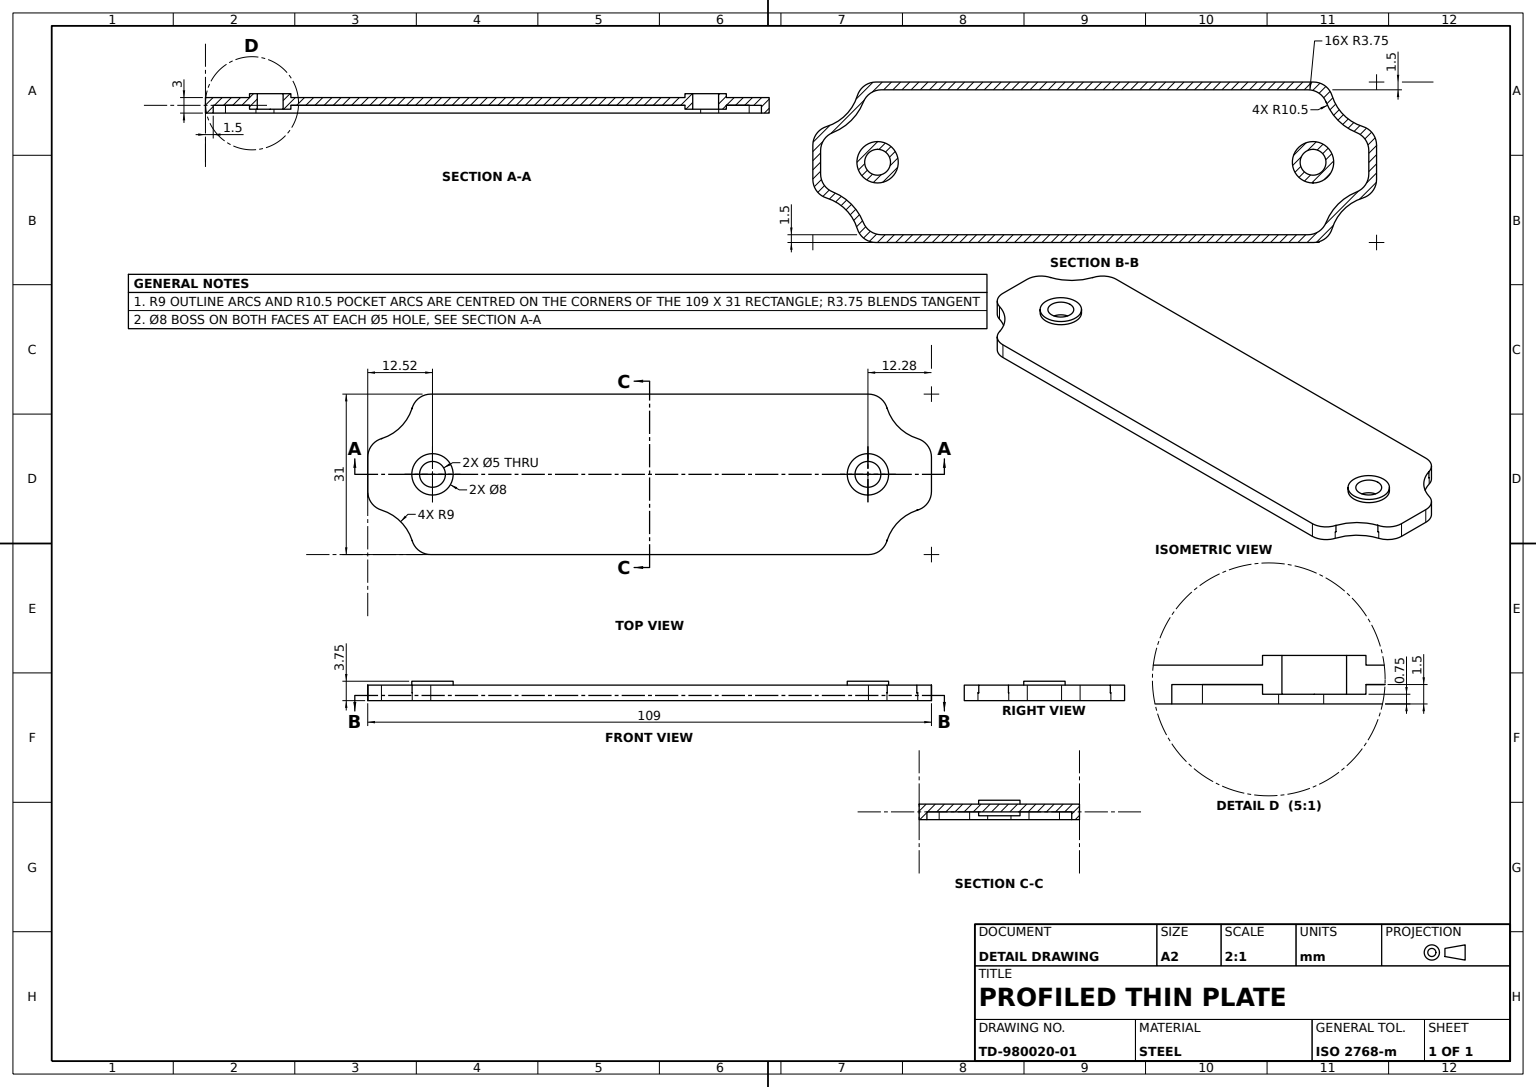
from build123d import *

# Parameters (mm, degrees)
PLATE_OUTLINE_SKETCH_R           = 2.5
BASE_PLATE_1_5MM_DEPTH           = 1.5
UNDERSIDE_BOSSES_DEPTH           = 3
THROUGH_START                    = -3
THROUGH_HOLES_DEPTH              = 3
RAISED_END_BOSS_B_8MM_DEPTH      = 0.75
RAISED_END_BOSS_B_8MM_DEPTH_BACK = 2.25
END_BOSS_B_SKETCH_R              = 4
END_BOSS_B_SKETCH_R_2            = 2.5
RAISED_END_BOSS_A_8MM_DEPTH      = 0.75
RAISED_END_BOSS_A_8MM_DEPTH_BACK = 2.25
END_BOSS_A_SKETCH_R              = 4
END_BOSS_A_SKETCH_R_2            = 2.5


with BuildPart() as part:
    # Plate Outline Sketch → Base Plate 1.5mm (new body)
    with BuildSketch(Plane(origin=(0, 0, 0), x_dir=(1, 0, 0), z_dir=(0, 1, 0))):
        with BuildLine():
            Line((-45.5, -15.5), (45.5, -15.5))
            ThreePointArc((45.5, -15.5), (48.136038969, -9.136038969), (54.5, -6.5))
            Line((54.5, -6.5), (54.5, 6.5))
            ThreePointArc((54.5, 6.5), (48.136038969, 9.136038969), (45.5, 15.5))
            Line((45.5, 15.5), (-45.5, 15.5))
            ThreePointArc((-45.5, 15.5), (-48.136038969, 9.136038969), (-54.5, 6.5))
            Line((-54.5, 6.5), (-54.5, -6.5))
            ThreePointArc((-54.5, -6.5), (-48.136038969, -9.136038969), (-45.5, -15.5))
        make_face()
        with Locations(Location((-41.982411865, 0, 0), (0, 0, 270))):
            Circle(PLATE_OUTLINE_SKETCH_R, mode=Mode.SUBTRACT)
        with Locations(Location((42.217053785, 0, 0), (0, 0, 270))):
            Circle(PLATE_OUTLINE_SKETCH_R, mode=Mode.SUBTRACT)
    extrude(amount=-BASE_PLATE_1_5MM_DEPTH)

    # Underside Boss Sketch → Underside Bosses (add)
    with BuildSketch(Plane(origin=(0, 0, 0), x_dir=(1, 0, 0), z_dir=(0, 1, 0))):
        with BuildLine():
            Line((42.313942393, 15.5), (-42.313942393, 15.5))
            ThreePointArc((-42.313942393, 15.5), (-44.541774365, 14.76649875), (-45.898076983, 12.852941176))
            ThreePointArc((-45.898076983, 12.852941176), (-48.136038969, 9.136038969), (-51.852941176, 6.898076983))
            ThreePointArc((-51.852941176, 6.898076983), (-53.76649875, 5.541774365), (-54.5, 3.313942393))
            Line((-54.5, 3.313942393), (-54.5, -3.313942393))
            ThreePointArc((-54.5, -3.313942393), (-53.76649875, -5.541774365), (-51.852941176, -6.898076983))
            ThreePointArc((-51.852941176, -6.898076983), (-48.136038969, -9.136038969), (-45.898076983, -12.852941176))
            ThreePointArc((-45.898076983, -12.852941176), (-44.541774365, -14.76649875), (-42.313942393, -15.5))
            Line((-42.313942393, -15.5), (42.313942393, -15.5))
            ThreePointArc((42.313942393, -15.5), (44.541774365, -14.76649875), (45.898076983, -12.852941176))
            ThreePointArc((45.898076983, -12.852941176), (48.136038969, -9.136038969), (51.852941176, -6.898076983))
            ThreePointArc((51.852941176, -6.898076983), (53.76649875, -5.541774365), (54.5, -3.313942393))
            Line((54.5, -3.313942393), (54.5, 3.313942393))
            ThreePointArc((54.5, 3.313942393), (53.76649875, 5.541774365), (51.852941176, 6.898076983))
            ThreePointArc((51.852941176, 6.898076983), (48.136038969, 9.136038969), (45.898076983, 12.852941176))
            ThreePointArc((45.898076983, 12.852941176), (44.541774365, 14.76649875), (42.313942393, 15.5))
        make_face()
        with BuildLine():
            Line((53, -2.252358701), (53, 2.252358701))
            ThreePointArc((53, 2.252358701), (52.35188822, 4.359676777), (50.631578947, 5.738580095))
            ThreePointArc((50.631578947, 5.738580095), (47.075378798, 8.075378798), (44.738580095, 11.631578947))
            ThreePointArc((44.738580095, 11.631578947), (43.359676777, 13.35188822), (41.252358701, 14))
            Line((41.252358701, 14), (-41.252358701, 14))
            ThreePointArc((-41.252358701, 14), (-43.359676777, 13.35188822), (-44.738580095, 11.631578947))
            ThreePointArc((-44.738580095, 11.631578947), (-47.075378798, 8.075378798), (-50.631578947, 5.738580095))
            ThreePointArc((-50.631578947, 5.738580095), (-52.35188822, 4.359676777), (-53, 2.252358701))
            Line((-53, 2.252358701), (-53, -2.252358701))
            ThreePointArc((-53, -2.252358701), (-52.35188822, -4.359676777), (-50.631578947, -5.738580095))
            ThreePointArc((-50.631578947, -5.738580095), (-47.075378798, -8.075378798), (-44.738580095, -11.631578947))
            ThreePointArc((-44.738580095, -11.631578947), (-43.359676777, -13.35188822), (-41.252358701, -14))
            Line((-41.252358701, -14), (41.252358701, -14))
            ThreePointArc((41.252358701, -14), (43.359676777, -13.35188822), (44.738580095, -11.631578947))
            ThreePointArc((44.738580095, -11.631578947), (47.075378798, -8.075378798), (50.631578947, -5.738580095))
            ThreePointArc((50.631578947, -5.738580095), (52.35188822, -4.359676777), (53, -2.252358701))
        make_face(mode=Mode.SUBTRACT)
    extrude(amount=-UNDERSIDE_BOSSES_DEPTH)

    # Through Hole Sketch → Through Holes (cut)
    with BuildSketch(Plane.XZ.offset(1.5).offset(THROUGH_START)):
        with BuildLine():
            Line((-42.313942393, 15.5), (-45.5, 15.5))
            Line((-45.5, 15.5), (-45.925158888, 12.760749931))
            ThreePointArc((-45.925158888, 12.760749931), (-44.580237581, 14.737709176), (-42.313942393, 15.5))
        make_face()
        with BuildLine():
            Line((42.313942393, 15.5), (45.5, 15.5))
            Line((45.5, 15.5), (45.95663868, 12.640653558))
            ThreePointArc((45.95663868, 12.640653558), (44.629385024, 14.699783962), (42.313942393, 15.5))
        make_face()
        with BuildLine():
            Line((54.5, 3.313942393), (54.5, 6.5))
            Line((54.5, 6.5), (51.587845302, 6.969146252))
            ThreePointArc((51.587845302, 6.969146252), (53.682952427, 5.650668748), (54.5, 3.313942393))
        make_face()
        with BuildLine():
            Line((51.852941176, -6.898076983), (54.5, -6.5))
            Line((54.5, -6.5), (54.5, -3.313942393))
            ThreePointArc((54.5, -3.313942393), (53.76649875, -5.541774365), (51.852941176, -6.898076983))
        make_face()
        with BuildLine():
            Line((42.313942393, -15.5), (45.5, -15.5))
            Line((45.5, -15.5), (45.936535538, -12.719184661))
            ThreePointArc((45.936535538, -12.719184661), (44.597367181, -14.724638001), (42.313942393, -15.5))
        make_face()
        with BuildLine():
            Line((-42.313942393, -15.5), (-45.5, -15.5))
            Line((-45.5, -15.5), (-45.950010453, -12.66733803))
            ThreePointArc((-45.950010453, -12.66733803), (-44.618555418, -14.708252661), (-42.313942393, -15.5))
        make_face()
        with BuildLine():
            Line((-54.5, -3.313942393), (-54.5, -6.5))
            Line((-54.5, -6.5), (-51.713850774, -6.937958354))
            ThreePointArc((-51.713850774, -6.937958354), (-53.722956475, -5.599556052), (-54.5, -3.313942393))
        make_face()
        with BuildLine():
            Line((-54.5, 3.313942393), (-54.5, 6.5))
            Line((-54.5, 6.5), (-51.852941176, 6.898076983))
            ThreePointArc((-51.852941176, 6.898076983), (-53.76649875, 5.541774365), (-54.5, 3.313942393))
        make_face()
    extrude(amount=THROUGH_HOLES_DEPTH, mode=Mode.SUBTRACT)

    # End Boss B Sketch → Raised End Boss B 8mm (add, two sides: drawn at the far end of the back side and taken through both)
    # profile 1 of 2: a face of its own
    with BuildSketch(Plane(origin=(0, 0, 0), x_dir=(1, 0, 0), z_dir=(0, 1, 0)).offset(-RAISED_END_BOSS_B_8MM_DEPTH_BACK)):
        with Locations(Location((-41.982411865, 0, 0), (0, 0, 270))):
            Circle(END_BOSS_B_SKETCH_R)
        with Locations(Location((-41.982411865, 0, 0), (0, 0, 270))):
            Circle(END_BOSS_B_SKETCH_R_2, mode=Mode.SUBTRACT)
    # profile 2 of 2: a face of its own
    with BuildSketch(Plane(origin=(0, 0, 0), x_dir=(1, 0, 0), z_dir=(0, 1, 0)).offset(-RAISED_END_BOSS_B_8MM_DEPTH_BACK)):
        with Locations(Location((42.217053785, 0, 0), (0, 0, 270))):
            Circle(END_BOSS_B_SKETCH_R)
        with Locations(Location((42.217053785, 0, 0), (0, 0, 270))):
            Circle(END_BOSS_B_SKETCH_R_2, mode=Mode.SUBTRACT)
    extrude(amount=RAISED_END_BOSS_B_8MM_DEPTH + RAISED_END_BOSS_B_8MM_DEPTH_BACK)

    # End Boss A Sketch → Raised End Boss A 8mm (add, two sides: drawn at the far end of the back side and taken through both)
    # profile 1 of 2: a face of its own
    with BuildSketch(Plane(origin=(0, 0, 0), x_dir=(1, 0, 0), z_dir=(0, 1, 0)).offset(-RAISED_END_BOSS_A_8MM_DEPTH_BACK)):
        with Locations(Location((-41.982411865, 0, 0), (0, 0, 270))):
            Circle(END_BOSS_A_SKETCH_R)
        with Locations(Location((-41.982411865, 0, 0), (0, 0, 270))):
            Circle(END_BOSS_A_SKETCH_R_2, mode=Mode.SUBTRACT)
    # profile 2 of 2: a face of its own
    with BuildSketch(Plane(origin=(0, 0, 0), x_dir=(1, 0, 0), z_dir=(0, 1, 0)).offset(-RAISED_END_BOSS_A_8MM_DEPTH_BACK)):
        with Locations(Location((42.217053785, 0, 0), (0, 0, 270))):
            Circle(END_BOSS_A_SKETCH_R)
        with Locations(Location((42.217053785, 0, 0), (0, 0, 270))):
            Circle(END_BOSS_A_SKETCH_R_2, mode=Mode.SUBTRACT)
    extrude(amount=RAISED_END_BOSS_A_8MM_DEPTH + RAISED_END_BOSS_A_8MM_DEPTH_BACK)


solid = part.part
